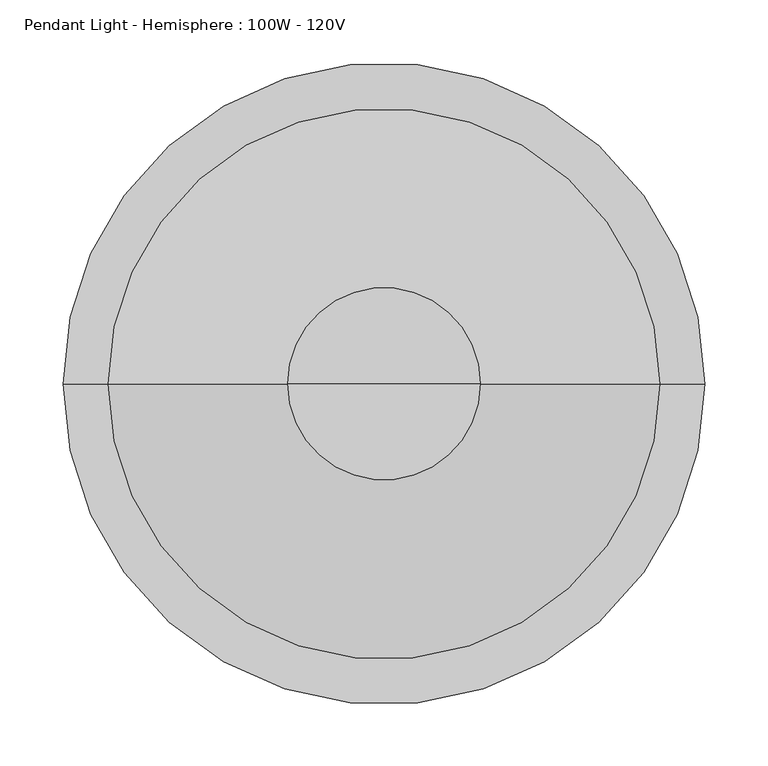
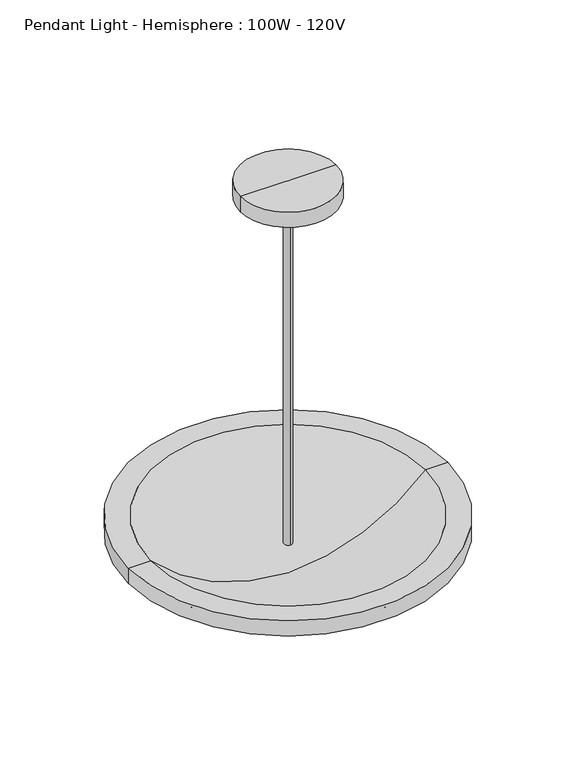
"""IFC4 building model written with IfcOpenShell, lengths in millimetres: light fixture geometry, Pendant Light - Hemisphere : 100W - 120V."""

from ifc_helpers import new_model, si_unit, point, frame, origin, place, context, project, spatial, polyline, circle_curve, ellipse_curve, trimmed, source, transform, mapped, element, save
from ifc_brep_helpers import plane_surface, cylinder_surface, revolved_surface, advanced_brep


def pendant_light_hemisphere_100w_120v_9c66a66f(model_context):
    return source(origin(), model_context, "Body", "AdvancedBrep", [
        advanced_brep(
        [(76.2, 0.0, 2413.0), (-76.2, 0.0, 2413.0), (-76.2, 0.0, 2438.4), (76.2, 0.0, 2438.4), (6.35, 0.0, 2380.4284101), (0.0, 6.35, 2380.4284101), (-6.35, 0.0, 2380.4284101), (0.0, -6.35, 2380.4284101), (-6.35, 0.0, 2438.4), (0.0, 0.0, 2438.4), (6.35, 0.0, 2438.4), (0.0, 6.35, 1828.8000062), (0.0, -6.35, 1828.8000062)],
        [
            (0, 1, circle_curve(frame((0.0, 0.0, 2413.0), z_axis=(0.0, 0.0, 1.0), x_axis=(-1.0, 0.0, 0.0)), 76.2)),
            (1, 2),
            (2, 3, circle_curve(frame((0.0, 0.0, 2438.4), z_axis=(0.0, 0.0, -1.0), x_axis=(-1.0, 0.0, 0.0)), 76.2)),
            (3, 0),
            (1, 0, circle_curve(frame((0.0, 0.0, 2413.0), z_axis=(0.0, 0.0, 1.0), x_axis=(-1.0, 0.0, 0.0)), 76.2)),
            (3, 2, circle_curve(frame((0.0, 0.0, 2438.4), z_axis=(0.0, 0.0, -1.0), x_axis=(-1.0, 0.0, 0.0)), 76.2)),
            (0, 4),
            (4, 5, circle_curve(frame((0.0, 0.0, 2380.4284101), z_axis=(0.0, 0.0, 1.0), x_axis=(-1.0, 0.0, 0.0)), 6.35)),
            (5, 6, circle_curve(frame((0.0, 0.0, 2380.4284101), z_axis=(0.0, 0.0, 1.0), x_axis=(-1.0, 0.0, 0.0)), 6.35)),
            (6, 1),
            (6, 7, circle_curve(frame((0.0, 0.0, 2380.4284101), z_axis=(0.0, 0.0, 1.0), x_axis=(-1.0, 0.0, 0.0)), 6.35)),
            (7, 4, circle_curve(frame((0.0, 0.0, 2380.4284101), z_axis=(0.0, 0.0, 1.0), x_axis=(-1.0, 0.0, 0.0)), 6.35)),
            (2, 8),
            (8, 9),
            (9, 10),
            (10, 3),
            (11, 12, circle_curve(frame((0.0, 0.0, 1828.8000062), z_axis=(0.0, 0.0, -1.0), x_axis=(0.0, -1.0, 0.0)), 6.35)),
            (12, 11, circle_curve(frame((0.0, 0.0, 1828.8000062), z_axis=(0.0, 0.0, -1.0), x_axis=(0.0, -1.0, 0.0)), 6.35)),
            (12, 7),
            (5, 11),
        ],
        [
            cylinder_surface(frame((0.0, 0.0, 2514.6), z_axis=(0.0, 0.0, -1.0), x_axis=(-1.0, 0.0, 0.0)), 76.2),
            revolved_surface(polyline([(-76.2, 0.0, 2413.0), (0.0, 0.0, 2377.4673564)]), (0.0, 0.0, 2514.6), (0.0, 0.0, -1.0)),
            plane_surface(frame((0.0, 0.0, 2438.4), z_axis=(0.0, 0.0, 1.0), x_axis=(-1.0, 0.0, 0.0))),
            plane_surface(frame((0.0, -6.35, 1828.8000062), z_axis=(0.0, 0.0, -1.0), x_axis=(-1.0, 0.0, 0.0))),
            cylinder_surface(frame((0.0, 0.0, 1828.8000062), z_axis=(0.0, 0.0, 1.0), x_axis=(0.0, -1.0, 0.0)), 6.35),
        ],
        [
            (0, [[1, 2, 3, 4]]),
            (0, [[-2, 5, -4, 6]]),
            (1, [[-1, 7, 8, 9, 10]]),
            (1, [[-5, -10, 11, 12, -7]]),
            (2, [[-3, 13, 14, 15, 16]]),
            (2, [[-6, -16, -15, -14, -13]]),
            (3, [[17, 18]]),
            (4, [[-18, 19, -11, -9, 20]]),
            (4, [[-17, -20, -8, -12, -19]]),
        ],
    ),
        advanced_brep(
        [(0.0, 0.0, 1752.5999938), (-228.9004272, 0.0, 1849.3282446), (228.9004272, 0.0, 1849.3282446), (218.3605921, 0.0, 1874.8510876), (-218.3605921, 0.0, 1874.8510876), (0.0, 0.0, 1777.9666257), (254.3004272, 0.0, 1874.8510876), (-254.3004272, 0.0, 1874.8510876), (254.3004272, 0.0, 1849.3282446), (-254.3004272, 0.0, 1849.3282446)],
        [
            (0, 1, circle_curve(frame((5.6276544, 0.0, 2085.1197309), z_axis=(0.0, 1.0, 0.0), x_axis=(0.0, 0.0, -1.0)), 332.5673556)),
            (1, 2, circle_curve(frame((0.0, 0.0, 1849.3282446), z_axis=(0.0, 0.0, -1.0), x_axis=(-1.0, 0.0, 0.0)), 228.9004272)),
            (2, 0, circle_curve(frame((-5.6276544, 0.0, 2085.1197309), z_axis=(0.0, 1.0, 0.0), x_axis=(0.0, 0.0, -1.0)), 332.5673556)),
            (2, 1, circle_curve(frame((0.0, 0.0, 1849.3282446), z_axis=(0.0, 0.0, -1.0), x_axis=(-1.0, 0.0, 0.0)), 228.9004272)),
            (3, 4, circle_curve(frame((0.0, 0.0, 1874.8510876), z_axis=(0.0, 0.0, 1.0), x_axis=(-1.0, 0.0, 0.0)), 218.3605921)),
            (4, 5, circle_curve(frame((7.2507854, 0.0, 2088.8241026), z_axis=(0.0, -1.0, 0.0), x_axis=(0.0, 0.0, -1.0)), 310.9420281)),
            (5, 3, circle_curve(frame((-7.2507854, 0.0, 2088.8241026), z_axis=(0.0, -1.0, 0.0), x_axis=(0.0, 0.0, -1.0)), 310.9420281)),
            (4, 3, circle_curve(frame((0.0, 0.0, 1874.8510876), z_axis=(0.0, 0.0, 1.0), x_axis=(-1.0, 0.0, 0.0)), 218.3605921)),
            (6, 7, circle_curve(frame((0.0, 0.0, 1874.8510876), z_axis=(0.0, 0.0, 1.0), x_axis=(-1.0, 0.0, 0.0)), 254.3004272)),
            (7, 4),
            (3, 6),
            (7, 6, circle_curve(frame((0.0, 0.0, 1874.8510876), z_axis=(0.0, 0.0, 1.0), x_axis=(-1.0, 0.0, 0.0)), 254.3004272)),
            (8, 9, circle_curve(frame((0.0, 0.0, 1849.3282446), z_axis=(0.0, 0.0, 1.0), x_axis=(-1.0, 0.0, 0.0)), 254.3004272)),
            (9, 7),
            (6, 8),
            (9, 8, circle_curve(frame((0.0, 0.0, 1849.3282446), z_axis=(0.0, 0.0, 1.0), x_axis=(-1.0, 0.0, 0.0)), 254.3004272)),
            (1, 9),
            (8, 2),
        ],
        [
            revolved_surface(trimmed(ellipse_curve(frame((5.6276544, 0.0, 2085.1197309), z_axis=(0.0, -1.0, 0.0), x_axis=(0.0, 0.0, -1.0)), 332.5673556, 332.5673556), [point((-228.9004272, 0.0, 1849.3282446))], [point((0.0, 0.0, 1752.5999938))], True, "CARTESIAN"), (0.0, 0.0, 1925.6510876), (0.0, 0.0, -1.0)),
            revolved_surface(trimmed(ellipse_curve(frame((7.2507854, 0.0, 2088.8241026), z_axis=(0.0, 1.0, 0.0), x_axis=(0.0, 0.0, -1.0)), 310.9420281, 310.9420281), [point((0.0, 0.0, 1777.9666257))], [point((-218.3605921, 0.0, 1874.8510876))], True, "CARTESIAN"), (0.0, 0.0, 1925.6510876), (0.0, 0.0, -1.0)),
            plane_surface(frame((0.0, 0.0, 1874.8510876), z_axis=(0.0, 0.0, 1.0), x_axis=(-1.0, 0.0, 0.0))),
            cylinder_surface(frame((0.0, 0.0, 1925.6510876), z_axis=(0.0, 0.0, -1.0), x_axis=(-1.0, 0.0, 0.0)), 254.3004272),
            plane_surface(frame((0.0, 0.0, 1849.3282446), z_axis=(0.0, 0.0, -1.0), x_axis=(-1.0, 0.0, 0.0))),
        ],
        [
            (0, [[1, 2, 3]]),
            (0, [[-3, 4, -1]]),
            (1, [[5, 6, 7]]),
            (1, [[8, -7, -6]]),
            (2, [[9, 10, -5, 11]]),
            (2, [[12, -11, -8, -10]]),
            (3, [[13, 14, -9, 15]]),
            (3, [[16, -15, -12, -14]]),
            (4, [[-2, 17, -13, 18]]),
            (4, [[-4, -18, -16, -17]]),
        ],
    ),
    ])


if __name__ == "__main__":
    model = new_model("IFC4")
    model_context = context("Model", 3, world=origin())
    ifc_project = project(units=[si_unit("LENGTHUNIT", "METRE", prefix="MILLI")], contexts=[model_context])
    site = spatial("IfcSite", under=ifc_project)
    building = spatial("IfcBuilding", under=site)
    placement = place(None, origin())
    pendant_light_hemisphere_100w_120v_shape = pendant_light_hemisphere_100w_120v_9c66a66f(model_context)
    element("IfcLightFixture", 1, ObjectType="Pendant Light - Hemisphere : 100W - 120V", at=placement, inside=building, context=model_context, shape_type="MappedRepresentation", body=[
        mapped(pendant_light_hemisphere_100w_120v_shape, transform((0.0, 0.0, 0.0), x_axis=(1.0, 0.0, 0.0), y_axis=(0.0, 1.0, 0.0), z_axis=(0.0, 0.0, 1.0))),
    ])
    save(model, "model.ifc")

# Revit data of these elements
# Type "Pendant Light - Hemisphere : 100W - 120V"
#   Lamp = "A-19"
#   Assembly Code = "D5020220"
#   Wattage = 100 W
#   built-in parameter 1150110 = 1 (stored number, unit not read)
#   built-in parameter 1114217 = 1 (stored number, unit not read)
#   built-in parameter 1150109 = 1 (stored number, unit not read)
#   built-in parameter 1150113 = 1 (stored number, unit not read)
#   built-in parameter 1150115 = 1 (stored number, unit not read)
#   built-in parameter 1150105 = 537.944 (stored number, unit not read)
#   Light Source Symbol Size = 2' - 0"
#   built-in parameter 1150112 = 1 (stored number, unit not read)
#   built-in parameter 1150114 = 1 (stored number, unit not read)
#   built-in parameter 1150107 = 2800 (stored number, unit not read)
#   built-in parameter 1150106 = 5.37944 (stored number, unit not read)
#   built-in parameter 1150104 = 1.57006 (stored number, unit not read)
#   Ballast Voltage = 120 V
#   built-in parameter 1114218 = 1 (stored number, unit not read)
#   built-in parameter 1150133 = 10 (stored number, unit not read)
#   Drop From Ceiling = 2' - 3"
#   Lumens = 1690 lm
#   Apparent Load = 100 VA
#   built-in parameter 1150134 = 4
#   built-in parameter 1150137 = 1
#   Color Filter = 16777215
#   built-in parameter 1140040 [instance default] = 1
#   Ballast Number of Poles = 1
#   Ceiling Mount Material = Steel, Chrome Plated
#   Pendant Material = Glass, Frosted
#   Dimming Lamp Color Temperature Shift = (empty or 0)
#   Default Elevation = 0
#   Wattage Comments = ""
# Element 1 (IfcLightFixture, "Pendant Light - Hemisphere : 100W - 120V")
#   Materials on its faces: "Glass, Frosted", "Steel, Chrome Plated"
# Materials
#   "Steel, Chrome Plated": class "Metal", colour RGB 17 17 17, transparency 0, Description = "Chromiuim plated steel", Cost = 0
#   "Glass, Frosted": class "Glass", colour RGB 250 244 225, transparency 0.55, Description = "physical material", Cost = 0
